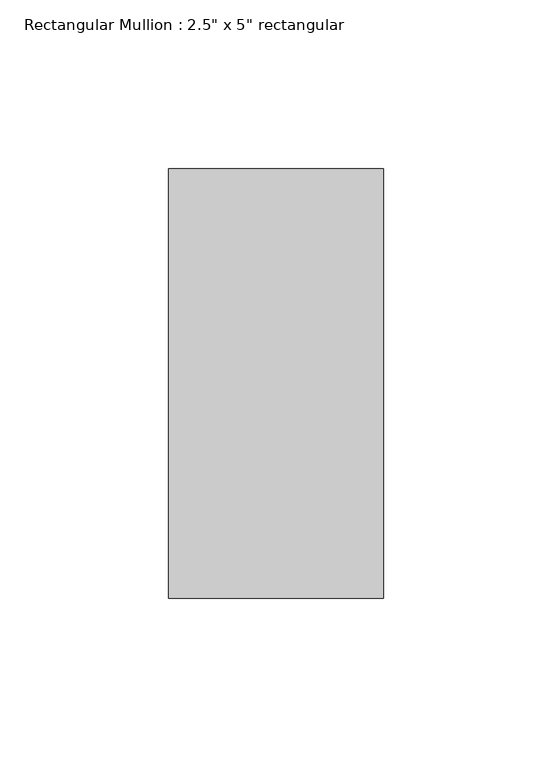
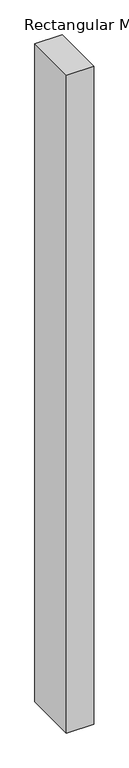
"""IFC4 building model written with IfcOpenShell, lengths in millimetres: member geometry."""

from ifc_helpers import new_model, si_unit, frame, origin, place, context, project, spatial, polyline, outline, extrude, source, transform, mapped, element, save


def member_74b724cb(model_context):
    return source(origin(), model_context, "Body", "SweptSolid", [
        extrude(outline(polyline([(31.75, 63.5), (31.75, -63.5), (-31.75, -63.5), (-31.75, 63.5), (31.75, 63.5)])), frame((0.0, 0.0, -1617.4100631), z_axis=(0.0, 0.0, 1.0), x_axis=(1.0, 0.0, 0.0)), (0.0, 0.0, 1.0), 1617.4100631),
    ])


if __name__ == "__main__":
    model = new_model("IFC4")
    model_context = context("Model", 3, world=origin())
    ifc_project = project(units=[si_unit("LENGTHUNIT", "METRE", prefix="MILLI")], contexts=[model_context])
    site = spatial("IfcSite", under=ifc_project)
    building = spatial("IfcBuilding", under=site)
    placement = place(None, origin())
    member_shape = member_74b724cb(model_context)
    element("IfcMember", 1, ObjectType="Rectangular Mullion : 2.5\" x 5\" rectangular", at=placement, inside=building, context=model_context, shape_type="MappedRepresentation", body=[
        mapped(member_shape, transform((0.0, 0.0, 0.0), x_axis=(1.0, 0.0, 0.0), y_axis=(0.0, 1.0, 0.0), z_axis=(0.0, 0.0, 1.0))),
    ])
    save(model, "model.ifc")

# Revit data of these elements
# Type "Rectangular Mullion : 2.5\" x 5\" rectangular"
#   built-in parameter 1007304 = 0.416667 (stored number, unit not read)
#   built-in parameter 1007301 = 0.104167 (stored number, unit not read)
#   built-in parameter 1007300 = 0.104167 (stored number, unit not read)
# Element 1 (IfcMember, "Rectangular Mullion : 2.5\" x 5\" rectangular")
#   Materials on its faces: "Aluminum"
# Materials
#   "Aluminum": class "Metal", colour RGB 247 247 247, transparency 0, Description = "Aluminum 6061", Cost = 0
